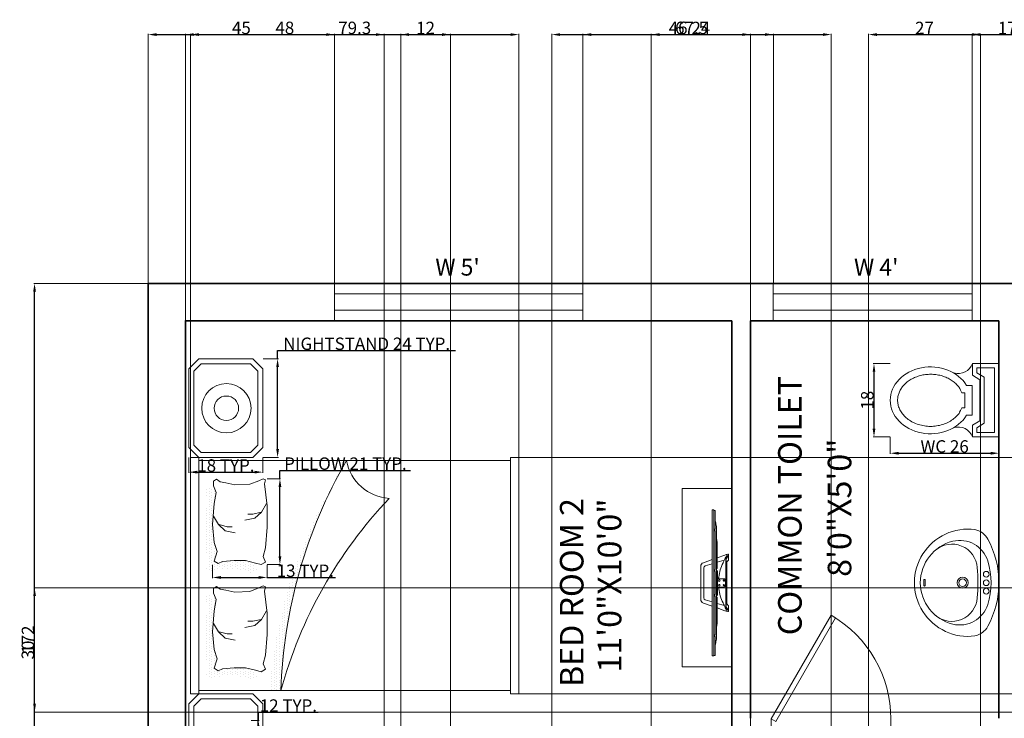
# Model space of a CAD drawing. Units: feet. Extents: x -297 to 770, y -228 to 625.
# Tile 7 of 14: x 351 to 589, y 202 to 371. Entities that reach past the tile are written whole.
import ezdxf

# ---------------------------------------------------------------- set-up
doc = ezdxf.new("R2010")
doc.units = ezdxf.units.FT
doc.header["$MEASUREMENT"] = 0
for name, color, linetype, lineweight in [('A-ANNO-DIMS', 2, 'Continuous', 18), ('A-ANNO-TEXT', 7, 'Continuous', 18), ('A-AREA-IDEN', 7, 'Continuous', 25), ('A-DETL-REFR', 8, 'Continuous', 13), ('A-EQPM', 8, 'Continuous', 13), ('A-FLOR-FIXT', 8, 'Continuous', 18), ('A-FURN', 8, 'Continuous', 18), ('A-FURN-PATT', 9, 'Continuous', 13), ('A-WALL', 7, 'Continuous', 35), ('doors', 30, 'Continuous', 18), ('Washbasin-detail', 251, 'Continuous', 13), ('Washbasin-outline', 250, 'Continuous', 18), ('windows', 30, 'Continuous', 18)]:
    doc.layers.add(name, color=color, linetype=linetype, lineweight=lineweight)
doc.styles.add('Annotative', font='arial.ttf')
doc.styles.get("Standard").update_dxf_attribs({"font": 'arial.ttf'})
doc.dimstyles.get("Standard").update_dxf_attribs({"dimtxt": 3, "dimasz": 2, "dimexe": 0.18, "dimexo": 0.0625, "dimgap": 0.09, "dimtad": 1, "dimtoh": 1, "dimdec": 1, "dimzin": 0, "dimdsep": 46, "dimlunit": 3, "dimtxsty": 'Standard', "dimcen": 0, "dimclre": 256, "dimadec": 0, "dimazin": 0, "dimtfac": 1, "dimtdec": 1, "dimtofl": 0, "dimtmove": 0, "dimatfit": 3, "dimfxl": 1, "dimtolj": 1, "dimtzin": 0, "dimlwe": -1, "dimarcsym": 0})
pattern_1 = [(90, (5458.5276, -7926.03606), (-0.629399927, 0.314699963), [0, -0.629399927])]

# ---------------------------------------------------------------- blocks, each defined once
blk = doc.blocks.new('*U3')
for p, q in [((0, 0), (0, -6)), ((40, 0), (40, -6))]:
    blk.add_line(p, q)
blk.add_lwpolyline([(0, 0), (20, 34.64), (21.52, 33.77), (1.52, -0.88)], close=True)
blk.add_arc((0, 0), 40, 0, 60)
blk = doc.blocks.new('A$C7C8779AE')
for p, q in [((0, 0.7405), (0, 0.5605)), ((0.5, 0.7405), (0, 0.7405)), ((0.5, 0.5605), (0.5, 0.7405)), ((0.47, 0.7105), (0.03, 0.7105)), ((0.03, 0.7105), (0.03, 0.5905)), ((0.47, 0.5905), (0.47, 0.7105)), ((0.093, 0.6405), (0.063, 0.5905)), ((0.11, 0.6105), (0.08, 0.5605)), ((0.093, 0.6405), (0.407, 0.6405)), ((0.11, 0.6105), (0.39, 0.6105)), ((0.42, 0.5605), (0.39, 0.6105)), ((0.437, 0.5905), (0.407, 0.6405)), ((0, 0.5605), (0.08, 0.5605)), ((0.03, 0.5905), (0.063, 0.5905)), ((0.1497, 0.557), (0.1497, 0.5203)), ((0.1497, 0.557), (0.3514, 0.557)), ((0.3514, 0.557), (0.3514, 0.5203)), ((0.42, 0.5605), (0.5, 0.5605)), ((0.437, 0.5905), (0.47, 0.5905)), ((0.1997, 0.507), (0.1997, 0.4879)), ((0.1997, 0.507), (0.3014, 0.507)), ((0.3014, 0.507), (0.3014, 0.4879))]:
    blk.add_line(p, q)
for centre, start, end in [((-0.0386, 0.4613), 344.64203, 68.73386), ((0.5386, 0.4613), 111.26614, 195.35797)]:
    blk.add_arc(centre, 0.1064, start, end)
blk.add_ellipse((0.2506, 0.2744), major_axis=(0, 0.2744), ratio=0.828948, start_param=0.459479, end_param=5.823706)
blk.add_open_spline([(0.1997, 0.4879), (0.1697, 0.474), (0.1642, 0.4702), (0.1512, 0.4602), (0.1438, 0.4535), (0.1298, 0.4388), (0.1233, 0.4306), (0.1111, 0.4131), (0.1055, 0.4037), (0.0956, 0.3838), (0.0912, 0.3733), (0.0838, 0.3516), (0.0808, 0.3403), (0.0762, 0.3172), (0.0746, 0.3055), (0.073, 0.2817), (0.0729, 0.2698), (0.0743, 0.246), (0.0758, 0.2342), (0.0801, 0.2111), (0.0831, 0.1998), (0.0903, 0.1779), (0.0945, 0.1673), (0.1043, 0.1473), (0.1098, 0.1378), (0.1218, 0.12), (0.1283, 0.1118), (0.1421, 0.0968), (0.1494, 0.09), (0.1646, 0.078), (0.1725, 0.0728), (0.1887, 0.064), (0.1969, 0.0603), (0.2137, 0.0547), (0.2222, 0.0527), (0.2392, 0.0502), (0.2478, 0.0498), (0.2664, 0.0505), (0.2764, 0.052), (0.2963, 0.0573), (0.3061, 0.061), (0.3253, 0.0707), (0.3346, 0.0766), (0.3525, 0.0906), (0.3611, 0.0987), (0.3771, 0.1169), (0.3845, 0.127), (0.3978, 0.1488), (0.4037, 0.1605), (0.4137, 0.1853), (0.4178, 0.1983), (0.424, 0.2251), (0.4261, 0.2389), (0.4282, 0.2668), (0.4283, 0.2809), (0.4262, 0.3088), (0.4241, 0.3226), (0.418, 0.3495), (0.414, 0.3625), (0.404, 0.3873), (0.3982, 0.3991), (0.385, 0.421), (0.3776, 0.4311), (0.3617, 0.4494), (0.3531, 0.4575), (0.3382, 0.4693), (0.3321, 0.4736), (0.3014, 0.4879)], degree=3, knots=[0.459479, 0.459479, 0.459479, 0.459479, 0.567422, 0.567422, 0.720865, 0.720865, 0.874307, 0.874307, 1.02775, 1.02775, 1.181192, 1.181192, 1.334635, 1.334635, 1.488077, 1.488077, 1.64152, 1.64152, 1.794963, 1.794963, 1.948405, 1.948405, 2.101848, 2.101848, 2.25529, 2.25529, 2.408733, 2.408733, 2.562175, 2.562175, 2.715618, 2.715618, 2.86906, 2.86906, 3.022503, 3.022503, 3.175946, 3.175946, 3.356457, 3.356457, 3.536968, 3.536968, 3.717479, 3.717479, 3.89799, 3.89799, 4.078501, 4.078501, 4.259012, 4.259012, 4.439523, 4.439523, 4.620035, 4.620035, 4.800546, 4.800546, 4.981057, 4.981057, 5.161568, 5.161568, 5.342079, 5.342079, 5.52259, 5.52259, 5.703101, 5.703101, 5.823706, 5.823706, 5.823706, 5.823706])
blk = doc.blocks.new('WIN-5FT')
for p, q in [((60, 6.5), (0, 6.5)), ((60, 2.5), (0, 2.5))]:
    blk.add_line(p, q)
blk.add_lwpolyline([(60, 0), (60, 9), (0, 9), (0, 0)], close=True)
blk = doc.blocks.new('WIN-4FT')
for p, q in [((48, 9), (0, 9)), ((0, 9), (0, 0)), ((48, 0), (48, 9)), ((0, 6.5), (48, 6.5)), ((0, 2.5), (48, 2.5)), ((0, 0), (48, 0))]:
    blk.add_line(p, q)
blk = doc.blocks.new('LAMP-BEDSIDE-ROUND')
for radius in [5.95, 2.95]:
    blk.add_circle((5.95, 5.95), radius)
blk = doc.blocks.new('NIGHTSTAND')
for points in [[(17.84, 2.38), (17.84, 21.41), (15.46, 23.79), (2.38, 23.79), (0, 21.41), (0, 2.38), (2.38, 0), (15.46, 0)], [(16.65, 2.97), (16.65, 20.81), (14.87, 22.6), (2.97, 22.6), (1.19, 20.81), (1.19, 2.97), (2.97, 1.19), (14.87, 1.19)]]:
    blk.add_lwpolyline(points, close=True)
blk = doc.blocks.new('BED-PILLOW')
for points in [[(1.1, 3.17), (0.37, 0.85), (1.34, 0.24), (2.44, 0.73), (5.24, 0.98), (7.92, 0.98), (10.36, 0.37), (11.7, 0), (12.8, 0.61), (12.19, 1.95), (12.8, 4.02), (13.16, 9.03), (13.16, 14.15), (12.55, 19.51), (12.8, 20.49), (12.19, 20.73), (11.21, 20.25), (9.02, 19.39), (5.36, 19.27), (3.17, 19.76), (1.83, 20), (0.97, 20.61), (0.24, 20.12), (0.24, 19.03), (0.85, 17.44), (0.37, 14.76), (0, 9.64), (0.37, 5.37), (1.1, 3.17)], [(13.04, 14.76), (11.82, 12.68), (10.24, 11.22), (7.8, 10.73)], [(11.7, 12.68), (9.75, 12.2), (8.53, 12.2)], [(0.24, 11.71), (1.46, 9.64), (3.05, 8.17), (5.48, 7.68)], [(1.58, 9.64), (3.53, 9.15), (4.75, 9.15)]]:
    blk.add_lwpolyline(points)
blk = doc.blocks.new('*D28')
at = {"layer": 'A-ANNO-DIMS', "color": 0, "lineweight": -2, "transparency": 16777216}
for p, q in [((408.77, 201.45), (408.77, 203.45)), ((408.77, 203.45), (423.18, 203.45)), ((408.77, 191.55), (408.77, 199.45))]:
    blk.add_line(p, q, dxfattribs=at)
at = {"layer": 'A-ANNO-DIMS', "transparency": 16777216}
for p, q in [((407.05, 201.45), (408.95, 201.45)), ((407.05, 189.55), (408.95, 189.55))]:
    blk.add_line(p, q, dxfattribs=at)
at = {"layer": 'A-ANNO-DIMS', "color": 0, "transparency": 16777216}
for points in [[(408.44, 199.45), (409.11, 199.45), (408.77, 201.45)], [(408.44, 191.55), (409.11, 191.55), (408.77, 189.55)]]:
    blk.add_solid(points, dxfattribs=at)
at = {"layer": 'Defpoints', "color": 0, "transparency": 16777216}
for p in [(406.99, 201.45), (408.77, 201.45), (406.99, 189.55)]:
    blk.add_point(p, dxfattribs=at)
at = {"layer": 'A-ANNO-DIMS', "color": 0, "transparency": 16777216, "insert": (416.02, 205.04), "char_height": 3, "attachment_point": 5}
blk.add_mtext('\\A1;12 TYP.', dxfattribs=at)
blk = doc.blocks.new('*D29')
at = {"layer": 'A-ANNO-DIMS', "color": 0, "lineweight": -2, "transparency": 16777216}
for p, q in [((413.41, 288.75), (413.41, 290.75)), ((413.41, 290.75), (456.36, 290.75)), ((413.41, 266.96), (413.41, 286.75))]:
    blk.add_line(p, q, dxfattribs=at)
at = {"layer": 'A-ANNO-DIMS', "transparency": 16777216}
for p, q in [((409.9, 288.75), (413.59, 288.75)), ((409.9, 264.96), (413.59, 264.96))]:
    blk.add_line(p, q, dxfattribs=at)
at = {"layer": 'A-ANNO-DIMS', "color": 0, "transparency": 16777216}
for points in [[(413.08, 286.75), (413.74, 286.75), (413.41, 288.75)], [(413.08, 266.96), (413.74, 266.96), (413.41, 264.96)]]:
    blk.add_solid(points, dxfattribs=at)
at = {"layer": 'Defpoints', "color": 0, "transparency": 16777216}
for p in [(409.84, 288.75), (413.41, 288.75), (409.84, 264.96)]:
    blk.add_point(p, dxfattribs=at)
at = {"layer": 'A-ANNO-DIMS', "color": 0, "transparency": 16777216, "insert": (434.93, 292.39), "char_height": 3, "attachment_point": 5}
blk.add_mtext('\\A1;NIGHTSTAND 24 TYP.', dxfattribs=at)
blk = doc.blocks.new('*D30')
at = {"layer": 'A-ANNO-DIMS', "transparency": 16777216}
for p, q in [((392, 264.9), (392, 261.21)), ((409.84, 264.9), (409.84, 261.21))]:
    blk.add_line(p, q, dxfattribs=at)
at = {"layer": 'A-ANNO-DIMS', "color": 0, "lineweight": -2, "transparency": 16777216}
blk.add_line((394, 261.39), (407.84, 261.39), dxfattribs=at)
at = {"layer": 'A-ANNO-DIMS', "color": 0, "transparency": 16777216}
for points in [[(394, 261.73), (394, 261.06), (392, 261.39)], [(407.84, 261.73), (407.84, 261.06), (409.84, 261.39)]]:
    blk.add_solid(points, dxfattribs=at)
at = {"layer": 'Defpoints', "color": 0, "transparency": 16777216}
for p in [(392, 264.96), (409.84, 264.96), (409.84, 261.39)]:
    blk.add_point(p, dxfattribs=at)
at = {"layer": 'A-ANNO-DIMS', "color": 0, "transparency": 16777216, "insert": (400.92, 263.01), "char_height": 3, "attachment_point": 5}
blk.add_mtext('\\A1;18 TYP.', dxfattribs=at)
blk = doc.blocks.new('*D31')
at = {"layer": 'A-ANNO-DIMS', "color": 0, "lineweight": -2, "transparency": 16777216}
for p, q in [((413.97, 259.81), (413.97, 261.81)), ((413.97, 261.81), (445.52, 261.81)), ((413.97, 241.08), (413.97, 257.81))]:
    blk.add_line(p, q, dxfattribs=at)
at = {"layer": 'A-ANNO-DIMS', "transparency": 16777216}
for p, q in [((410.93, 259.81), (414.15, 259.81)), ((410.93, 239.08), (414.15, 239.08))]:
    blk.add_line(p, q, dxfattribs=at)
at = {"layer": 'A-ANNO-DIMS', "color": 0, "transparency": 16777216}
for points in [[(413.64, 257.81), (414.31, 257.81), (413.97, 259.81)], [(413.64, 241.08), (414.31, 241.08), (413.97, 239.08)]]:
    blk.add_solid(points, dxfattribs=at)
at = {"layer": 'Defpoints', "color": 0, "transparency": 16777216}
for p in [(410.86, 259.81), (413.97, 259.81), (410.86, 239.08)]:
    blk.add_point(p, dxfattribs=at)
at = {"layer": 'A-ANNO-DIMS', "color": 0, "transparency": 16777216, "insert": (429.79, 263.45), "char_height": 3, "attachment_point": 5}
blk.add_mtext('\\A1;PILLOW 21 TYP.', dxfattribs=at)
blk = doc.blocks.new('*D32')
at = {"layer": 'A-ANNO-DIMS', "transparency": 16777216}
for p, q in [((397.7, 239.02), (397.7, 235.79)), ((410.86, 239.02), (410.86, 235.79))]:
    blk.add_line(p, q, dxfattribs=at)
at = {"layer": 'A-ANNO-DIMS', "color": 0, "lineweight": -2, "transparency": 16777216}
for p, q in [((399.7, 235.97), (408.86, 235.97)), ((410.86, 235.97), (427.36, 235.97))]:
    blk.add_line(p, q, dxfattribs=at)
at = {"layer": 'A-ANNO-DIMS', "color": 0, "transparency": 16777216}
for points in [[(399.7, 236.3), (399.7, 235.63), (397.7, 235.97)], [(408.86, 236.3), (408.86, 235.63), (410.86, 235.97)]]:
    blk.add_solid(points, dxfattribs=at)
at = {"layer": 'Defpoints', "color": 0, "transparency": 16777216}
for p in [(397.7, 239.08), (410.86, 239.08), (410.86, 235.97)]:
    blk.add_point(p, dxfattribs=at)
at = {"layer": 'A-ANNO-DIMS', "color": 0, "transparency": 16777216, "insert": (420.11, 237.59), "char_height": 3, "attachment_point": 5}
blk.add_mtext('\\A1;13 TYP.', dxfattribs=at)
blk = doc.blocks.new('*D37')
at = {"layer": 'A-ANNO-DIMS', "transparency": 16777216}
for p, q in [((561.41, 269.83), (561.41, 265.78)), ((587.66, 269.83), (587.66, 265.78))]:
    blk.add_line(p, q, dxfattribs=at)
at = {"layer": 'A-ANNO-DIMS', "color": 0, "lineweight": -2, "transparency": 16777216}
blk.add_line((563.41, 265.96), (585.66, 265.96), dxfattribs=at)
at = {"layer": 'A-ANNO-DIMS', "color": 0, "transparency": 16777216}
for points in [[(563.41, 266.29), (563.41, 265.62), (561.41, 265.96)], [(585.66, 266.29), (585.66, 265.62), (587.66, 265.96)]]:
    blk.add_solid(points, dxfattribs=at)
at = {"layer": 'Defpoints', "color": 0, "transparency": 16777216}
for p in [(561.41, 269.89), (587.66, 269.89), (587.66, 265.96)]:
    blk.add_point(p, dxfattribs=at)
at = {"layer": 'A-ANNO-DIMS', "color": 0, "transparency": 16777216, "insert": (574.53, 267.6), "char_height": 3, "attachment_point": 5}
blk.add_mtext('\\A1;WC 26', dxfattribs=at)
blk = doc.blocks.new('*D38')
at = {"layer": 'A-ANNO-DIMS', "transparency": 16777216}
for p, q in [((561.34, 287.62), (557.29, 287.62)), ((561.34, 269.89), (557.29, 269.89))]:
    blk.add_line(p, q, dxfattribs=at)
at = {"layer": 'A-ANNO-DIMS', "color": 0, "lineweight": -2, "transparency": 16777216}
blk.add_line((557.47, 285.62), (557.47, 271.89), dxfattribs=at)
at = {"layer": 'A-ANNO-DIMS', "color": 0, "transparency": 16777216}
for points in [[(557.14, 285.62), (557.8, 285.62), (557.47, 287.62)], [(557.14, 271.89), (557.8, 271.89), (557.47, 269.89)]]:
    blk.add_solid(points, dxfattribs=at)
at = {"layer": 'Defpoints', "color": 0, "transparency": 16777216}
for p in [(561.41, 287.62), (557.47, 269.89), (561.41, 269.89)]:
    blk.add_point(p, dxfattribs=at)
at = {"layer": 'A-ANNO-DIMS', "color": 0, "transparency": 16777216, "insert": (555.85, 278.76), "char_height": 3, "attachment_point": 5, "rotation": 90}
blk.add_mtext('\\A1;18', dxfattribs=at)
blk = doc.blocks.new('*D46')
at = {"layer": 'A-ANNO-DIMS', "transparency": 16777216}
for p, q in [((382.16, 307.03), (382.16, 367.22)), ((427.16, 307.03), (427.16, 367.22))]:
    blk.add_line(p, q, dxfattribs=at)
at = {"layer": 'A-ANNO-DIMS', "color": 0, "lineweight": -2, "transparency": 16777216}
blk.add_line((384.16, 367.04), (425.16, 367.04), dxfattribs=at)
at = {"layer": 'A-ANNO-DIMS', "color": 0, "transparency": 16777216}
for points in [[(384.16, 367.38), (384.16, 366.71), (382.16, 367.04)], [(425.16, 367.38), (425.16, 366.71), (427.16, 367.04)]]:
    blk.add_solid(points, dxfattribs=at)
at = {"layer": 'Defpoints', "color": 0, "transparency": 16777216}
for p in [(427.16, 367.04), (382.16, 306.96), (427.16, 306.96)]:
    blk.add_point(p, dxfattribs=at)
at = {"layer": 'A-ANNO-DIMS', "color": 0, "transparency": 16777216, "insert": (404.66, 368.66), "char_height": 3, "attachment_point": 5}
blk.add_mtext('\\A1;45', dxfattribs=at)
blk = doc.blocks.new('*D47')
at = {"layer": 'A-ANNO-DIMS', "transparency": 16777216}
for p, q in [((487.16, 307.03), (487.16, 367.22)), ((533.16, 307.03), (533.16, 367.22))]:
    blk.add_line(p, q, dxfattribs=at)
at = {"layer": 'A-ANNO-DIMS', "color": 0, "lineweight": -2, "transparency": 16777216}
blk.add_line((489.16, 367.04), (531.16, 367.04), dxfattribs=at)
at = {"layer": 'A-ANNO-DIMS', "color": 0, "transparency": 16777216}
for points in [[(489.16, 367.38), (489.16, 366.71), (487.16, 367.04)], [(531.16, 367.38), (531.16, 366.71), (533.16, 367.04)]]:
    blk.add_solid(points, dxfattribs=at)
at = {"layer": 'Defpoints', "color": 0, "transparency": 16777216}
for p in [(533.16, 367.04), (487.16, 306.96), (533.16, 306.96)]:
    blk.add_point(p, dxfattribs=at)
at = {"layer": 'A-ANNO-DIMS', "color": 0, "transparency": 16777216, "insert": (510.16, 368.66), "char_height": 3, "attachment_point": 5}
blk.add_mtext('\\A1;46', dxfattribs=at)
blk = doc.blocks.new('*D48')
at = {"layer": 'A-ANNO-DIMS', "transparency": 16777216}
for p, q in [((581.16, 307.03), (581.16, 367.22)), ((598.16, 307.03), (598.16, 367.22))]:
    blk.add_line(p, q, dxfattribs=at)
at = {"layer": 'A-ANNO-DIMS', "color": 0, "lineweight": -2, "transparency": 16777216}
blk.add_line((583.16, 367.04), (596.16, 367.04), dxfattribs=at)
at = {"layer": 'A-ANNO-DIMS', "color": 0, "transparency": 16777216}
for points in [[(583.16, 367.38), (583.16, 366.71), (581.16, 367.04)], [(596.16, 367.38), (596.16, 366.71), (598.16, 367.04)]]:
    blk.add_solid(points, dxfattribs=at)
at = {"layer": 'Defpoints', "color": 0, "transparency": 16777216}
for p in [(598.16, 367.04), (581.16, 306.96), (598.16, 306.96)]:
    blk.add_point(p, dxfattribs=at)
at = {"layer": 'A-ANNO-DIMS', "color": 0, "transparency": 16777216, "insert": (589.66, 368.64), "char_height": 3, "attachment_point": 5}
blk.add_mtext('\\A1;17', dxfattribs=at)
blk = doc.blocks.new('*D51')
at = {"layer": 'A-ANNO-DIMS', "transparency": 16777216}
for p, q in [((382.09, 306.96), (354.53, 306.96)), ((382.09, 134.96), (354.53, 134.96))]:
    blk.add_line(p, q, dxfattribs=at)
at = {"layer": 'A-ANNO-DIMS', "color": 0, "lineweight": -2, "transparency": 16777216}
blk.add_line((354.71, 136.96), (354.71, 304.96), dxfattribs=at)
at = {"layer": 'A-ANNO-DIMS', "color": 0, "transparency": 16777216}
for points in [[(354.37, 304.96), (355.04, 304.96), (354.71, 306.96)], [(354.37, 136.96), (355.04, 136.96), (354.71, 134.96)]]:
    blk.add_solid(points, dxfattribs=at)
at = {"layer": 'Defpoints', "color": 0, "transparency": 16777216}
for p in [(354.71, 306.96), (382.16, 306.96), (382.16, 134.96)]:
    blk.add_point(p, dxfattribs=at)
at = {"layer": 'A-ANNO-DIMS', "color": 0, "transparency": 16777216, "insert": (353.11, 220.96), "char_height": 3, "attachment_point": 5, "rotation": 90}
blk.add_mtext('\\A1;172', dxfattribs=at)
blk = doc.blocks.new('*D54')
at = {"layer": 'A-ANNO-DIMS', "transparency": 16777216}
for p, q in [((733.1, 233.46), (354.53, 233.46)), ((733.09, 203.46), (354.53, 203.46))]:
    blk.add_line(p, q, dxfattribs=at)
at = {"layer": 'A-ANNO-DIMS', "color": 0, "lineweight": -2, "transparency": 16777216}
blk.add_line((354.71, 205.46), (354.71, 231.46), dxfattribs=at)
at = {"layer": 'A-ANNO-DIMS', "color": 0, "transparency": 16777216}
for points in [[(354.37, 231.46), (355.04, 231.46), (354.71, 233.46)], [(354.37, 205.46), (355.04, 205.46), (354.71, 203.46)]]:
    blk.add_solid(points, dxfattribs=at)
at = {"layer": 'Defpoints', "color": 0, "transparency": 16777216}
for p in [(354.71, 233.46), (733.16, 233.46), (733.16, 203.46)]:
    blk.add_point(p, dxfattribs=at)
at = {"layer": 'A-ANNO-DIMS', "color": 0, "transparency": 16777216, "insert": (353.08, 218.46), "char_height": 3, "attachment_point": 5, "rotation": 90}
blk.add_mtext('\\A1;30', dxfattribs=at)
blk = doc.blocks.new('*D57')
at = {"layer": 'A-ANNO-DIMS', "transparency": 16777216}
for p, q in [((391.16, -163.97), (391.16, 367.22)), ((439.16, -163.97), (439.16, 367.22))]:
    blk.add_line(p, q, dxfattribs=at)
at = {"layer": 'A-ANNO-DIMS', "color": 0, "lineweight": -2, "transparency": 16777216}
blk.add_line((393.16, 367.04), (437.16, 367.04), dxfattribs=at)
at = {"layer": 'A-ANNO-DIMS', "color": 0, "transparency": 16777216}
for points in [[(393.16, 367.38), (393.16, 366.71), (391.16, 367.04)], [(437.16, 367.38), (437.16, 366.71), (439.16, 367.04)]]:
    blk.add_solid(points, dxfattribs=at)
at = {"layer": 'Defpoints', "color": 0, "transparency": 16777216}
for p in [(439.16, 367.04), (391.16, -164.04), (439.16, -164.04)]:
    blk.add_point(p, dxfattribs=at)
at = {"layer": 'A-ANNO-DIMS', "color": 0, "transparency": 16777216, "insert": (415.16, 368.66), "char_height": 3, "attachment_point": 5}
blk.add_mtext('\\A1;48', dxfattribs=at)
blk = doc.blocks.new('*D60')
at = {"layer": 'A-ANNO-DIMS', "transparency": 16777216}
for p, q in [((556.16, -144.47), (556.16, 367.22)), ((583.16, -144.47), (583.16, 367.22))]:
    blk.add_line(p, q, dxfattribs=at)
at = {"layer": 'A-ANNO-DIMS', "color": 0, "lineweight": -2, "transparency": 16777216}
blk.add_line((558.16, 367.04), (581.16, 367.04), dxfattribs=at)
at = {"layer": 'A-ANNO-DIMS', "color": 0, "transparency": 16777216}
for points in [[(558.16, 367.38), (558.16, 366.71), (556.16, 367.04)], [(581.16, 367.38), (581.16, 366.71), (583.16, 367.04)]]:
    blk.add_solid(points, dxfattribs=at)
at = {"layer": 'Defpoints', "color": 0, "transparency": 16777216}
for p in [(583.16, 367.04), (556.16, -144.54), (583.16, -144.54)]:
    blk.add_point(p, dxfattribs=at)
at = {"layer": 'A-ANNO-DIMS', "color": 0, "transparency": 16777216, "insert": (569.66, 368.64), "char_height": 3, "attachment_point": 5}
blk.add_mtext('\\A1;27', dxfattribs=at)
blk = doc.blocks.new('*D66')
at = {"layer": 'A-ANNO-DIMS', "transparency": 16777216}
for p, q in [((503.66, 125.53), (503.66, 367.22)), ((527.66, 125.53), (527.66, 367.22))]:
    blk.add_line(p, q, dxfattribs=at)
at = {"layer": 'A-ANNO-DIMS', "color": 0, "lineweight": -2, "transparency": 16777216}
blk.add_line((505.66, 367.04), (525.66, 367.04), dxfattribs=at)
at = {"layer": 'A-ANNO-DIMS', "color": 0, "transparency": 16777216}
for points in [[(505.66, 367.38), (505.66, 366.71), (503.66, 367.04)], [(525.66, 367.38), (525.66, 366.71), (527.66, 367.04)]]:
    blk.add_solid(points, dxfattribs=at)
at = {"layer": 'Defpoints', "color": 0, "transparency": 16777216}
for p in [(527.66, 367.04), (503.66, 125.46), (527.66, 125.46)]:
    blk.add_point(p, dxfattribs=at)
at = {"layer": 'A-ANNO-DIMS', "color": 0, "transparency": 16777216, "insert": (515.66, 368.64), "char_height": 3, "attachment_point": 5}
blk.add_mtext('\\A1;24', dxfattribs=at)
blk = doc.blocks.new('*D72')
at = {"layer": 'A-ANNO-DIMS', "transparency": 16777216}
for p, q in [((479.66, 49.03), (479.66, 367.22)), ((547.16, 49.03), (547.16, 367.22))]:
    blk.add_line(p, q, dxfattribs=at)
at = {"layer": 'A-ANNO-DIMS', "color": 0, "lineweight": -2, "transparency": 16777216}
blk.add_line((481.66, 367.04), (545.16, 367.04), dxfattribs=at)
at = {"layer": 'A-ANNO-DIMS', "color": 0, "transparency": 16777216}
for points in [[(481.66, 367.38), (481.66, 366.71), (479.66, 367.04)], [(545.16, 367.38), (545.16, 366.71), (547.16, 367.04)]]:
    blk.add_solid(points, dxfattribs=at)
at = {"layer": 'Defpoints', "color": 0, "transparency": 16777216}
for p in [(547.16, 367.04), (479.66, 48.96), (547.16, 48.96)]:
    blk.add_point(p, dxfattribs=at)
at = {"layer": 'A-ANNO-DIMS', "color": 0, "transparency": 16777216, "insert": (513.41, 368.66), "char_height": 3, "attachment_point": 5}
blk.add_mtext('\\A1;67.5', dxfattribs=at)
blk = doc.blocks.new('*D74')
at = {"layer": 'A-ANNO-DIMS', "transparency": 16777216}
for p, q in [((392.4, 265.02), (392.4, 367.22)), ((471.69, 265.02), (471.69, 367.22))]:
    blk.add_line(p, q, dxfattribs=at)
at = {"layer": 'A-ANNO-DIMS', "color": 0, "lineweight": -2, "transparency": 16777216}
blk.add_line((394.4, 367.04), (469.69, 367.04), dxfattribs=at)
at = {"layer": 'A-ANNO-DIMS', "color": 0, "transparency": 16777216}
for points in [[(394.4, 367.38), (394.4, 366.71), (392.4, 367.04)], [(469.69, 367.38), (469.69, 366.71), (471.69, 367.04)]]:
    blk.add_solid(points, dxfattribs=at)
at = {"layer": 'Defpoints', "color": 0, "transparency": 16777216}
for p in [(471.69, 367.04), (392.4, 264.96), (471.69, 264.96)]:
    blk.add_point(p, dxfattribs=at)
at = {"layer": 'A-ANNO-DIMS', "color": 0, "transparency": 16777216, "insert": (432.04, 368.66), "char_height": 3, "attachment_point": 5}
blk.add_mtext('\\A1;79.3', dxfattribs=at)
blk = doc.blocks.new('*D75')
at = {"layer": 'A-ANNO-DIMS', "transparency": 16777216}
for p, q in [((471.75, 264.96), (769.79, 264.96)), ((471.75, 207.87), (769.79, 207.87))]:
    blk.add_line(p, q, dxfattribs=at)
at = {"layer": 'A-ANNO-DIMS', "color": 0, "lineweight": -2, "transparency": 16777216}
blk.add_line((769.61, 209.87), (769.61, 262.96), dxfattribs=at)
at = {"layer": 'A-ANNO-DIMS', "color": 0, "transparency": 16777216}
for points in [[(769.27, 262.96), (769.94, 262.96), (769.61, 264.96)], [(769.27, 209.87), (769.94, 209.87), (769.61, 207.87)]]:
    blk.add_solid(points, dxfattribs=at)
at = {"layer": 'Defpoints', "color": 0, "transparency": 16777216}
for p in [(471.69, 264.96), (769.61, 264.96), (471.69, 207.87)]:
    blk.add_point(p, dxfattribs=at)
at = {"layer": 'A-ANNO-DIMS', "color": 0, "transparency": 16777216, "insert": (767.98, 236.42), "char_height": 3, "attachment_point": 5, "rotation": 90}
blk.add_mtext('\\A1;57.09', dxfattribs=at)
blk = doc.blocks.new('*D76')
at = {"layer": 'A-ANNO-DIMS', "transparency": 16777216}
for p, q in [((443.16, 89.53), (443.16, 367.22)), ((455.16, 89.53), (455.16, 367.22))]:
    blk.add_line(p, q, dxfattribs=at)
at = {"layer": 'A-ANNO-DIMS', "color": 0, "lineweight": -2, "transparency": 16777216}
blk.add_line((445.16, 367.04), (453.16, 367.04), dxfattribs=at)
at = {"layer": 'A-ANNO-DIMS', "color": 0, "transparency": 16777216}
for points in [[(445.16, 367.38), (445.16, 366.71), (443.16, 367.04)], [(453.16, 367.38), (453.16, 366.71), (455.16, 367.04)]]:
    blk.add_solid(points, dxfattribs=at)
at = {"layer": 'Defpoints', "color": 0, "transparency": 16777216}
for p in [(455.16, 367.04), (443.16, 89.46), (455.16, 89.46)]:
    blk.add_point(p, dxfattribs=at)
at = {"layer": 'A-ANNO-DIMS', "color": 0, "transparency": 16777216, "insert": (449.16, 368.64), "char_height": 3, "attachment_point": 5}
blk.add_mtext('\\A1;12', dxfattribs=at)

msp = doc.modelspace()

# ---------------------------------------------------------------- hatches: boundary and pattern name
at = {"layer": 'A-FURN-PATT'}
h = msp.add_hatch(dxfattribs=at)
h.set_pattern_fill('DOTS', color=256, scale=0.396472, angle=90, style=0)
h.set_pattern_definition(pattern_1)
h.paths.add_polyline_path([(411.483, 208.662), (414.202, 208.662, -0.1242731), (430.061, 264.168, 0.1225633)])
h = msp.add_hatch(dxfattribs=at)
h.set_pattern_fill('DOTS', color=256, scale=0.396472, angle=90, style=0)
h.set_pattern_definition(pattern_1)
h.paths.add_polyline_path([(396.7, 231.809), (395.969, 231.321), (395.969, 230.223), (396.578, 228.638), (396.09, 225.955), (395.725, 220.832), (396.09, 216.564), (396.822, 214.368), (396.09, 212.051), (397.065, 211.441), (398.162, 211.929), (400.965, 212.173), (403.646, 212.173), (406.083, 211.563), (407.423, 211.197), (408.52, 211.807), (407.911, 213.149), (408.029, 213.551), (405.623, 214.153), (402.942, 214.153), (400.139, 213.909), (399.042, 213.421), (398.068, 214.031), (398.799, 216.348), (398.068, 218.543), (397.702, 222.812), (398.068, 227.934), (398.555, 230.618), (398.39, 231.047), (397.553, 231.199)])
h.paths.add_polyline_path([(396.7, 257.71), (395.969, 257.222), (395.969, 256.125), (396.578, 254.539), (396.09, 251.856), (395.725, 246.734), (396.09, 242.465), (396.822, 240.27), (396.09, 237.952), (397.065, 237.343), (398.162, 237.83), (400.965, 238.074), (403.646, 238.074), (406.083, 237.464), (407.423, 237.099), (408.52, 237.708), (407.911, 239.05), (408.029, 239.452), (405.623, 240.054), (402.942, 240.054), (400.139, 239.81), (399.042, 239.322), (398.068, 239.932), (398.799, 242.249), (398.068, 244.445), (397.702, 248.713), (398.068, 253.836), (398.555, 256.519), (398.39, 256.948), (397.553, 257.1)])

# ---------------------------------------------------------------- linework, layer by layer
at = {"layer": 'A-DETL-REFR'}
msp.add_line((487.298, 212.232), (487.298, 212.232), dxfattribs=at)
at = {"layer": 'A-EQPM'}
for p, q in [((518.41, 252.197), (518.41, 234.647)), ((518.746, 252.298), (518.51, 252.298)), ((518.746, 252.172), (518.746, 252.298)), ((518.746, 252.172), (518.746, 234.661)), ((519.006, 252.172), (518.746, 252.172)), ((519.106, 250.005), (519.106, 252.072)), ((519.106, 250.005), (519.106, 247.765)), ((518.947, 247.421), (518.947, 247.46)), ((518.947, 247.421), (518.947, 247.382)), ((518.987, 247.271), (518.987, 247.571)), ((519.403, 248.29), (519.403, 234.661)), ((519.106, 247.076), (519.106, 237.999)), ((519.583, 239.588), (519.583, 244.34)), ((518.41, 240.3), (516.263, 239.537)), ((521.438, 241.375), (519.583, 240.716)), ((521.555, 240.661), (521.555, 240.661)), ((521.693, 240.473), (521.693, 234.661)), ((522.315, 241.428), (521.745, 240.617)), ((521.765, 240.47), (521.765, 234.661)), ((522.347, 241.35), (521.803, 240.576)), ((522.329, 241.382), (522.329, 241.382)), ((522.347, 240.341), (522.347, 241.35)), ((515.616, 238.643), (515.616, 234.661)), ((516.358, 234.661), (516.358, 238.261)), ((516.696, 238.764), (518.41, 239.276)), ((519.403, 238.072), (519.451, 238.072)), ((519.583, 239.626), (519.625, 239.638)), ((519.583, 238.176), (519.583, 239.588)), ((519.625, 239.638), (521.264, 240.147)), ((519.625, 239.638), (519.625, 239.638)), ((521.914, 234.661), (521.914, 239.59)), ((521.955, 239.712), (522.295, 240.175)), ((518.947, 237.655), (518.947, 237.693)), ((518.947, 237.655), (518.947, 237.616)), ((518.987, 237.505), (518.987, 237.805)), ((519.106, 237.31), (519.106, 234.661)), ((519.477, 237.682), (519.403, 237.682)), ((519.669, 237.568), (519.477, 237.682)), ((519.695, 234.661), (519.695, 237.507)), ((519.956, 235.867), (519.695, 235.887)), ((521.336, 235.602), (519.695, 235.671)), ((519.93, 235.661), (519.981, 236.072)), ((515.616, 230.679), (515.616, 234.661)), ((516.358, 234.661), (516.358, 231.061)), ((518.41, 217.124), (518.41, 234.674)), ((518.746, 217.149), (518.746, 234.661)), ((519.106, 232.011), (519.106, 234.661)), ((519.403, 221.031), (519.403, 234.661)), ((519.695, 234.661), (519.695, 231.814)), ((521.336, 233.72), (519.695, 233.65)), ((519.956, 233.455), (519.695, 233.434)), ((519.93, 233.66), (519.981, 233.249)), ((521.607, 234.661), (521.607, 235.295)), ((521.607, 234.661), (521.607, 234.661)), ((521.607, 234.661), (521.607, 234.026)), ((521.607, 234.661), (521.607, 234.661)), ((521.693, 228.849), (521.693, 234.661)), ((521.765, 228.852), (521.765, 234.661)), ((521.914, 234.661), (521.914, 229.732)), ((518.947, 231.667), (518.947, 231.706)), ((518.947, 231.667), (518.947, 231.628)), ((518.987, 231.817), (518.987, 231.517)), ((519.106, 222.245), (519.106, 231.323)), ((519.477, 231.64), (519.403, 231.64)), ((519.403, 231.249), (519.451, 231.249)), ((519.669, 231.753), (519.477, 231.64)), ((519.583, 231.145), (519.583, 229.734)), ((518.41, 229.022), (516.263, 229.784)), ((516.696, 230.558), (518.41, 230.046)), ((519.583, 229.734), (519.583, 224.982)), ((519.583, 229.696), (519.625, 229.683)), ((521.438, 227.946), (519.583, 228.605)), ((519.625, 229.683), (519.625, 229.683)), ((519.625, 229.683), (521.264, 229.174)), ((521.555, 228.661), (521.555, 228.661)), ((522.315, 227.893), (521.745, 228.704)), ((522.347, 227.972), (521.803, 228.746)), ((521.955, 229.609), (522.295, 229.147)), ((522.347, 228.98), (522.347, 227.972)), ((522.329, 227.94), (522.329, 227.94)), ((518.947, 221.901), (518.947, 221.94)), ((518.947, 221.901), (518.947, 221.862)), ((518.987, 222.051), (518.987, 221.751)), ((519.106, 219.317), (519.106, 221.556)), ((519.106, 219.317), (519.106, 217.25)), ((518.746, 217.024), (518.51, 217.024)), ((519.006, 217.149), (518.746, 217.149)), ((518.746, 217.149), (518.746, 217.024))]:
    msp.add_line(p, q, dxfattribs=at)
for centre, radius in [((520.107, 235.219), 0.192), ((520.107, 234.102), 0.192), ((521.204, 235.219), 0.173), ((521.204, 234.102), 0.173)]:
    msp.add_circle(centre, radius, dxfattribs=at)
for centre, radius, start, end in [((518.51, 252.197), 0.1, 90, 180), ((519.006, 252.072), 0.1, 0, 90), ((522.384, 250.184), 3.283, 183.13295, 193.15331), ((519.122, 247.46), 0.175, 132.05139, 180), ((519.122, 247.382), 0.175, 180, 227.94861), ((518.743, 247.879), 0.39, 312.05139, 331.65405), ((518.94, 247.773), 0.166, 331.65405, 357.30713), ((475.085, 239.131), 45.291, 12.48046, 13.15331), ((514.476, 247.849), 4.947, 5.11021, 12.48046), ((518.743, 246.962), 0.39, 28.34595, 47.94861), ((518.94, 247.069), 0.166, 2.69287, 28.34595), ((517.09, 244.34), 2.493, 0, 21.90061), ((480.583, 258.941), 44.865, 334.27627, 335.95504), ((522.925, 237.114), 4.513, 105.03026, 109.23595), ((537.091, 230.816), 18.392, 145.81308, 147.63909), ((521.979, 240.453), 0.286, 144.88854, 175.98923), ((522.624, 238.237), 3.351, 97.75527, 105.03026), ((521.979, 240.453), 0.214, 144.88854, 175.36433), ((521.806, 241.195), 0.0833, 327.98819, 40.32248), ((522.194, 241.394), 0.165, 46.41299, 97.75527), ((522.08, 240.333), 0.267, 323.62537, 1.66061), ((522.257, 241.466), 0.069, 327.05691, 43.25595), ((522.442, 241.442), 0.128, 186.03725, 207.91075), ((522.526, 241.473), 0.217, 204.7304, 214.57256), ((516.589, 238.62), 0.974, 109.55394, 178.64567), ((516.902, 238.261), 0.543, 112.2689, 180), ((518.743, 238.113), 0.39, 312.05139, 331.65405), ((518.94, 238.007), 0.166, 331.65405, 357.30713), ((519.45, 238.209), 0.136, 270.17438, 346.17499), ((530.552, 234.747), 10.653, 153.69355, 172.8538), ((521.276, 240.11), 0.0391, 24.56662, 107.24388), ((522.12, 239.59), 0.206, 143.49658, 180), ((519.122, 237.693), 0.175, 132.05139, 180), ((519.122, 237.616), 0.175, 180, 227.94861), ((518.743, 237.196), 0.39, 28.34595, 47.94861), ((518.94, 237.302), 0.166, 2.69287, 28.34595), ((519.609, 237.507), 0.0853, 0, 45.39175), ((521.313, 235.308), 0.294, 357.46685, 85.45225), ((530.552, 234.575), 10.653, 187.1462, 206.30645), ((521.313, 234.013), 0.294, 274.54775, 2.53315), ((516.902, 231.061), 0.543, 180, 247.7311), ((519.122, 231.706), 0.175, 132.05139, 180), ((519.122, 231.628), 0.175, 180, 227.94861), ((518.743, 232.125), 0.39, 312.05139, 331.65405), ((518.743, 231.209), 0.39, 28.34595, 47.94861), ((518.94, 232.019), 0.166, 331.65405, 357.30713), ((518.94, 231.315), 0.166, 2.69287, 28.34595), ((519.45, 231.113), 0.136, 13.82501, 89.82562), ((519.609, 231.814), 0.0853, 314.60825, 0), ((516.589, 230.702), 0.974, 181.35433, 250.44606), ((480.583, 210.381), 44.865, 24.04496, 25.72373), ((521.276, 229.212), 0.0391, 252.75612, 335.43338), ((537.091, 238.505), 18.392, 212.36091, 214.18692), ((521.979, 228.869), 0.286, 184.01077, 215.11146), ((521.979, 228.869), 0.214, 184.63567, 215.11146), ((522.12, 229.732), 0.206, 180, 216.50342), ((522.08, 228.988), 0.267, 358.33939, 36.37463), ((522.925, 232.207), 4.513, 250.76405, 254.96974), ((522.624, 231.085), 3.351, 254.96974, 262.24473), ((521.806, 228.127), 0.0833, 319.67752, 32.01181), ((522.194, 227.928), 0.165, 262.24473, 313.58701), ((522.257, 227.856), 0.069, 316.74405, 32.94309), ((522.442, 227.88), 0.128, 152.08925, 173.96275), ((522.526, 227.849), 0.217, 145.42744, 155.2696), ((517.09, 224.982), 2.493, 338.09939, 0), ((519.122, 221.94), 0.175, 132.05139, 180), ((519.122, 221.862), 0.175, 180, 227.94861), ((518.743, 222.359), 0.39, 312.05139, 331.65405), ((518.743, 221.442), 0.39, 28.34595, 47.94861), ((518.94, 222.253), 0.166, 331.65405, 357.30713), ((518.94, 221.549), 0.166, 2.69287, 28.34595), ((522.384, 219.137), 3.283, 166.84669, 176.86705), ((475.085, 230.191), 45.291, 346.84669, 347.51954), ((514.476, 221.472), 4.947, 347.51954, 354.88979), ((518.51, 217.124), 0.1, 180, 270), ((519.006, 217.25), 0.1, 270, 0)]:
    msp.add_arc(centre, radius, start, end, dxfattribs=at)
at = {"layer": 'A-FURN'}
for p, q in [((392.396, 264.961), (392.396, 207.869)), ((392.396, 264.961), (394.378, 264.961)), ((394.378, 264.961), (394.378, 207.869)), ((394.378, 264.168), (469.708, 264.168)), ((469.708, 264.961), (469.708, 207.869)), ((469.708, 264.961), (471.691, 264.961)), ((471.691, 264.961), (471.691, 207.869)), ((523.155, 257.415), (511.155, 257.415)), ((511.155, 257.415), (511.155, 214.415)), ((523.155, 214.415), (523.155, 257.415)), ((511.155, 214.415), (523.155, 214.415)), ((394.378, 207.869), (392.396, 207.869)), ((469.708, 208.662), (394.378, 208.662)), ((471.691, 207.869), (469.708, 207.869))]:
    msp.add_line(p, q, dxfattribs=at)
for centre, radius, start, end in [((532.069, 205.004), 117.923, 149.8866, 178.22261), ((440.995, 266.166), 11.115, 190.35432, 266.78617), ((519.368, 179.938), 109.018, 136.43667, 164.72336)]:
    msp.add_arc(centre, radius, start, end, dxfattribs=at)
at = {"layer": 'A-WALL'}
for p, q in [((523.155, 197.463), (523.155, 297.963)), ((527.655, 201.963), (527.655, 297.963)), ((587.655, 201.963), (587.655, 297.963))]:
    msp.add_line(p, q, dxfattribs=at)
for points in [[(685.155, 306.963), (382.155, 306.963), (382.155, -173.037), (556.155, -173.037)], [(523.155, 297.963), (391.155, 297.963), (391.155, 177.963)], [(587.655, 297.963), (527.655, 297.963)]]:
    msp.add_lwpolyline(points, dxfattribs=at)
at = {"layer": 'Washbasin-detail'}
for p, q in [((569.513, 235.36), (569.513, 234.696)), ((569.513, 234.031), (569.513, 234.696)), ((569.816, 235.36), (569.816, 234.696)), ((569.816, 234.031), (569.816, 234.696))]:
    msp.add_line(p, q, dxfattribs=at)
for centre, radius in [((578.878, 234.696), 1.327), ((578.878, 234.696), 0.919), ((584.593, 236.737), 0.694), ((584.593, 234.696), 0.694), ((584.593, 232.655), 0.694)]:
    msp.add_circle(centre, radius, dxfattribs=at)
for centre, radius, start, end in [((576.282, 237.878), 6.143, 4.57625, 130.13804), ((536.522, 234.696), 46.031, 355.42376, 4.57625), ((569.664, 235.36), 0.152, 0, 180), ((569.664, 234.031), 0.152, 180, 0), ((576.282, 231.513), 6.143, 229.86196, 355.42376)]:
    msp.add_arc(centre, radius, start, end, dxfattribs=at)
at = {"layer": 'Washbasin-outline'}
for centre, radius, start, end in [((580.205, 234.696), 12.962, 82.63359, 277.36642), ((580.813, 242.945), 4.725, 28.79365, 77.11194), ((565.804, 234.696), 21.851, 331.20636, 28.79365), ((578.966, 234.696), 10.305, 103.79872, 256.20128), ((578.199, 237.821), 7.088, 17.43481, 103.79872), ((568.248, 234.696), 17.517, 342.56519, 17.43481), ((578.199, 231.571), 7.088, 256.20128, 342.56519), ((580.813, 226.447), 4.725, 282.88807, 331.20636)]:
    msp.add_arc(centre, radius, start, end, dxfattribs=at)

# ---------------------------------------------------------------- block references
at = {"layer": 'A-FLOR-FIXT', "xscale": 35.44919325486015, "yscale": 35.44919325486015, "zscale": 35.44919325486015, "rotation": 270}
msp.add_blockref('A$C7C8779AE', (561.406, 287.618), dxfattribs=at)
at = {"layer": 'A-FURN'}
for name, p in [('NIGHTSTAND', (392, 264.961)), ('LAMP-BEDSIDE-ROUND', (395.094, 270.876)), ('BED-PILLOW', (397.702, 239.078)), ('BED-PILLOW', (397.702, 213.177)), ('NIGHTSTAND', (392, 184.081))]:
    msp.add_blockref(name, p, dxfattribs=at)
at = {"layer": 'doors', "xscale": 0.7226421799388985, "yscale": 0.7226421799388985, "zscale": 0.7226421799388985}
msp.add_blockref('*U3', (532.655, 201.799), dxfattribs=at)
at = {"layer": 'windows'}
for name, p in [('WIN-5FT', (427.155, 297.963)), ('WIN-4FT', (533.155, 297.963))]:
    msp.add_blockref(name, p, dxfattribs=at)

# ---------------------------------------------------------------- texts
at = {"layer": 'A-ANNO-TEXT', "style": 'Annotative'}
for s, p in [("W 5'", (451.518, 308.849)), ("W 4'", (552.654, 308.849))]:
    msp.add_text(s, height=4.0626, dxfattribs=at).set_placement(p)
at = {"layer": 'A-AREA-IDEN', "style": 'Annotative'}
for s, height, p in [('COMMON TOILET', 5.69601, (540.005, 222.012)), ('8\'0"X5\'0"', 5.696, (551.993, 236.115)), ('BED ROOM 2', 5.696, (487.298, 209.533)), ('  11\'0"X10\'0"', 5.69601, (496.448, 209.533))]:
    msp.add_text(s, height=height, rotation=90, dxfattribs=at).set_placement(p)

# ---------------------------------------------------------------- dimensions: what is measured, and where the dimension line sits
at = {"layer": 'A-ANNO-DIMS'}
for base, p1, p2, override, picture, middle in [((427.155, 367.042), (382.155, 306.963), (427.155, 306.963), {"dimdec": 0, "dimlfac": 1, "dimrnd": 0, "dimzin": 0, "dimdsep": 46, "dimlunit": 2}, '*D46', (404.655, 368.658)), ((439.155, 367.042), (391.155, -164.037), (439.155, -164.037), {"dimdec": 0, "dimlfac": 1, "dimrnd": 0, "dimzin": 0, "dimdsep": 46, "dimlunit": 2}, '*D57', (415.155, 368.664)), ((471.691, 367.042), (392.396, 264.961), (471.691, 264.961), {"dimdec": 1, "dimlfac": 1, "dimrnd": 0, "dimzin": 0, "dimdsep": 46, "dimlunit": 2}, '*D74', (432.043, 368.665)), ((455.155, 367.042), (443.155, 89.463), (455.155, 89.463), {"dimdec": 0, "dimlfac": 1, "dimrnd": 0, "dimzin": 0, "dimdsep": 46, "dimlunit": 2}, '*D76', (449.155, 368.638)), ((547.155, 367.042), (479.655, 48.963), (547.155, 48.963), {"dimdec": 1, "dimlfac": 1, "dimrnd": 0, "dimzin": 0, "dimdsep": 46, "dimlunit": 2}, '*D72', (513.405, 368.664)), ((533.155, 367.042), (487.155, 306.963), (533.155, 306.963), {"dimdec": 0, "dimlfac": 1, "dimrnd": 0, "dimzin": 0, "dimdsep": 46, "dimlunit": 2}, '*D47', (510.155, 368.664)), ((527.655, 367.042), (503.655, 125.463), (527.655, 125.463), {"dimdec": 0, "dimlfac": 1, "dimrnd": 0, "dimzin": 0, "dimdsep": 46, "dimlunit": 2}, '*D66', (515.655, 368.638)), ((583.155, 367.042), (556.155, -144.537), (583.155, -144.537), {"dimdec": 0, "dimlfac": 1, "dimrnd": 0, "dimzin": 0, "dimdsep": 46, "dimlunit": 2}, '*D60', (569.655, 368.638)), ((598.155, 367.042), (581.155, 306.963), (598.155, 306.963), {"dimdec": 0, "dimlfac": 1, "dimrnd": 0, "dimzin": 0, "dimdsep": 46, "dimlunit": 2}, '*D48', (589.655, 368.638))]:
    dim = msp.add_linear_dim(base=base, p1=p1, p2=p2, dimstyle='Standard', override=override, dxfattribs=at)
    dim.commit()
    dim.dimension.update_dxf_attribs({"geometry": picture, "text_midpoint": middle})
for base, p1, p2, angle, override, picture, middle in [((354.705, 306.963), (382.155, 134.963), (382.155, 306.963), 90, {"dimdec": 0, "dimlfac": 1, "dimrnd": 0, "dimzin": 0, "dimdsep": 46, "dimlunit": 2}, '*D51', (353.109, 220.963)), ((557.469, 269.894), (561.406, 287.618), (561.406, 269.894), 270, {"dimdec": 0, "dimlfac": 1, "dimrnd": 0, "dimzin": 0, "dimdsep": 46, "dimlunit": 2}, '*D38', (555.847, 278.756)), ((769.605, 264.961), (471.691, 207.869), (471.691, 264.961), 90, {"dimdec": 2, "dimlfac": 1, "dimrnd": 0, "dimzin": 0, "dimdsep": 46, "dimlunit": 2}, '*D75', (767.984, 236.415)), ((354.705, 233.463), (733.155, 203.463), (733.158, 233.463), 90, {"dimdec": 0, "dimlfac": 1, "dimrnd": 0, "dimzin": 0, "dimdsep": 46, "dimlunit": 2}, '*D54', (353.083, 218.463))]:
    dim = msp.add_linear_dim(base=base, p1=p1, p2=p2, angle=angle, dimstyle='Standard', override=override, dxfattribs=at)
    dim.commit()
    dim.dimension.update_dxf_attribs({"geometry": picture, "text_midpoint": middle})
for base, p1, p2, text, picture, middle in [((413.409, 288.749), (409.841, 264.961), (409.841, 288.749), 'NIGHTSTAND <> TYP.', '*D29', (434.931, 292.391)), ((413.973, 259.812), (410.863, 239.078), (410.863, 259.812), 'PILLOW <> TYP.', '*D31', (429.79, 263.454)), ((408.772, 201.447), (406.988, 189.552), (406.988, 201.447), '<> TYP.', '*D28', (416.023, 205.044))]:
    dim = msp.add_linear_dim(base=base, p1=p1, p2=p2, angle=90, text=text, dimstyle='Standard', override={"dimdec": 0, "dimlfac": 1, "dimrnd": 0, "dimzin": 0, "dimdsep": 46, "dimlunit": 2}, dxfattribs=at)
    dim.commit()
    dim.dimension.update_dxf_attribs({"geometry": picture, "text_midpoint": middle})
for base, p1, p2, text, picture, middle in [((587.655, 265.957), (561.406, 269.894), (587.655, 269.894), 'WC <>', '*D37', (574.531, 267.598)), ((409.841, 261.393), (392, 264.961), (409.841, 264.961), '<> TYP.', '*D30', (400.92, 263.015)), ((410.863, 235.968), (397.702, 239.078), (410.863, 239.078), '<> TYP.', '*D32', (420.113, 237.591))]:
    dim = msp.add_linear_dim(base=base, p1=p1, p2=p2, text=text, dimstyle='Standard', override={"dimdec": 0, "dimlfac": 1, "dimrnd": 0, "dimzin": 0, "dimdsep": 46, "dimlunit": 2}, dxfattribs=at)
    dim.commit()
    dim.dimension.update_dxf_attribs({"geometry": picture, "text_midpoint": middle})

doc.saveas('drawing.dxf')
